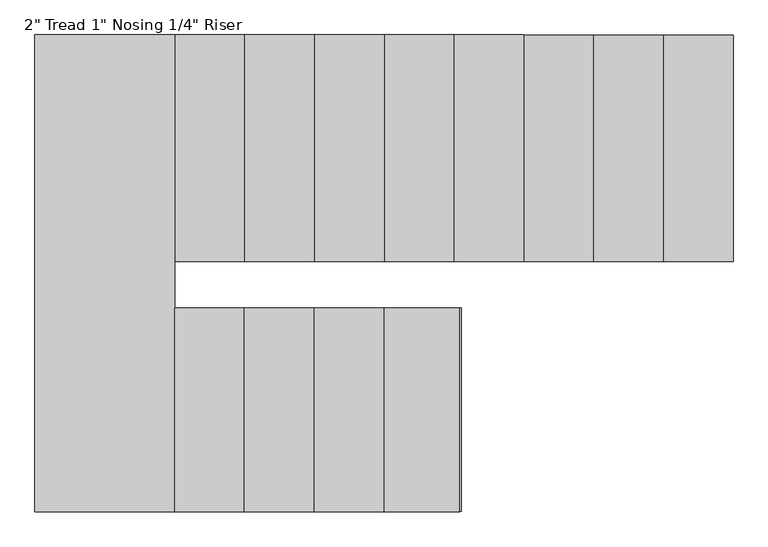
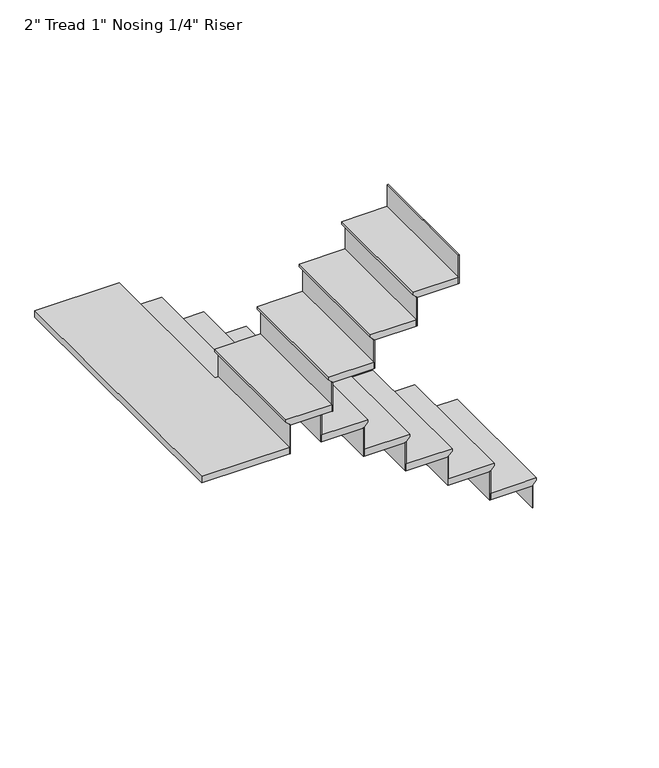
"""IFC4 building model written with IfcOpenShell, lengths in millimetres: stair flight geometry."""

from ifc_helpers import new_model, si_unit, origin, place, context, project, spatial, faceted_brep, source, transform, mapped, element, save


def stair_flight_46f16e2a(model_context):
    return source(origin(), model_context, "Body", "Brep", [
        faceted_brep([(-569.5630704, 657.3457979, 198.6642857), (-569.5630704, 657.3457979, 217.7142857), (-569.5630704, -333.2542021, 217.7142857), (-569.5630704, -333.2542021, 198.6642857), (-594.9630704, 657.3457979, 173.2642857), (-594.9630704, -333.2542021, 173.2642857), (-899.7630704, 657.3457979, 217.7142857), (-899.7630704, -333.2542021, 217.7142857), (-594.9630704, -333.2542021, 166.9142857), (-899.7630704, -333.2542021, 166.9142857), (-899.7630704, 657.3457979, 166.9142857), (-594.9630704, 657.3457979, 166.9142857)], [[[0, 1, 2, 3]], [[4, 0, 3, 5]], [[2, 1, 6, 7]], [[8, 9, 10, 11]], [[2, 7, 9, 8, 5, 3]], [[8, 11, 4, 5]], [[6, 1, 0, 4, 11, 10]], [[7, 6, 10, 9]]]),
        faceted_brep([(-594.9630704, 657.3457979, 166.9142857), (-594.9630704, 657.3457979, 0.0), (-601.3130704, 657.3457979, 0.0), (-601.3130704, 657.3457979, 166.9142857), (-594.9630704, -333.2542021, 166.9142857), (-601.3130704, -333.2542021, 166.9142857), (-601.3130704, -333.2542021, 0.0), (-594.9630704, -333.2542021, 0.0)], [[[0, 1, 2, 3]], [[4, 5, 6, 7]], [[1, 0, 4, 7]], [[2, 1, 7, 6]], [[3, 2, 6, 5]], [[0, 3, 5, 4]]]),
        faceted_brep([(-899.7630704, 657.3457979, 384.6285714), (-899.7630704, 657.3457979, 166.9142857), (-906.1130704, 657.3457979, 166.9142857), (-906.1130704, 657.3457979, 384.6285714), (-899.7630704, -333.2542021, 384.6285714), (-906.1130704, -333.2542021, 384.6285714), (-906.1130704, -333.2542021, 166.9142857), (-899.7630704, -333.2542021, 166.9142857)], [[[0, 1, 2, 3]], [[4, 5, 6, 7]], [[1, 0, 4, 7]], [[2, 1, 7, 6]], [[3, 2, 6, 5]], [[0, 3, 5, 4]]]),
        faceted_brep([(-874.3630704, -333.2542021, 435.4285714), (-874.3630704, 657.3457979, 435.4285714), (-1204.5630704, 657.3457979, 435.4285714), (-1204.5630704, -333.2542021, 435.4285714), (-899.7630704, -333.2542021, 384.6285714), (-1204.5630704, -333.2542021, 384.6285714), (-1204.5630704, 657.3457979, 384.6285714), (-899.7630704, 657.3457979, 384.6285714), (-899.7630704, -333.2542021, 390.9785714), (-874.3630704, -333.2542021, 416.3785714), (-899.7630704, 657.3457979, 390.9785714), (-874.3630704, 657.3457979, 416.3785714)], [[[0, 1, 2, 3]], [[4, 5, 6, 7]], [[0, 3, 5, 4, 8, 9]], [[4, 7, 10, 8]], [[2, 1, 11, 10, 7, 6]], [[3, 2, 6, 5]], [[11, 1, 0, 9]], [[10, 11, 9, 8]]]),
        faceted_brep([(-1204.5630704, 657.3457979, 602.3428571), (-1204.5630704, 657.3457979, 384.6285714), (-1210.9130704, 657.3457979, 384.6285714), (-1210.9130704, 657.3457979, 602.3428571), (-1204.5630704, -333.2542021, 602.3428571), (-1210.9130704, -333.2542021, 602.3428571), (-1210.9130704, -333.2542021, 384.6285714), (-1204.5630704, -333.2542021, 384.6285714)], [[[0, 1, 2, 3]], [[4, 5, 6, 7]], [[1, 0, 4, 7]], [[2, 1, 7, 6]], [[3, 2, 6, 5]], [[0, 3, 5, 4]]]),
        faceted_brep([(-1179.1630704, -333.2542021, 653.1428571), (-1179.1630704, 657.3457979, 653.1428571), (-1509.3630704, 657.3457979, 653.1428571), (-1509.3630704, -333.2542021, 653.1428571), (-1204.5630704, -333.2542021, 602.3428571), (-1509.3630704, -333.2542021, 602.3428571), (-1509.3630704, 657.3457979, 602.3428571), (-1204.5630704, 657.3457979, 602.3428571), (-1204.5630704, -333.2542021, 608.6928571), (-1179.1630704, -333.2542021, 634.0928571), (-1204.5630704, 657.3457979, 608.6928571), (-1179.1630704, 657.3457979, 634.0928571)], [[[0, 1, 2, 3]], [[4, 5, 6, 7]], [[0, 3, 5, 4, 8, 9]], [[4, 7, 10, 8]], [[2, 1, 11, 10, 7, 6]], [[3, 2, 6, 5]], [[11, 1, 0, 9]], [[10, 11, 9, 8]]]),
        faceted_brep([(-1509.3630704, 657.3457979, 820.0571429), (-1509.3630704, 657.3457979, 602.3428571), (-1515.7130704, 657.3457979, 602.3428571), (-1515.7130704, 657.3457979, 820.0571429), (-1509.3630704, -333.2542021, 820.0571429), (-1515.7130704, -333.2542021, 820.0571429), (-1515.7130704, -333.2542021, 602.3428571), (-1509.3630704, -333.2542021, 602.3428571)], [[[0, 1, 2, 3]], [[4, 5, 6, 7]], [[1, 0, 4, 7]], [[2, 1, 7, 6]], [[3, 2, 6, 5]], [[0, 3, 5, 4]]]),
        faceted_brep([(-1483.9630704, -333.2542021, 870.8571429), (-1483.9630704, 657.3457979, 870.8571429), (-1814.1630704, 657.3457979, 870.8571429), (-1814.1630704, -333.2542021, 870.8571429), (-1509.3630704, -333.2542021, 820.0571429), (-1814.1630704, -333.2542021, 820.0571429), (-1814.1630704, 657.3457979, 820.0571429), (-1509.3630704, 657.3457979, 820.0571429), (-1509.3630704, -333.2542021, 826.4071429), (-1483.9630704, -333.2542021, 851.8071429), (-1509.3630704, 657.3457979, 826.4071429), (-1483.9630704, 657.3457979, 851.8071429)], [[[0, 1, 2, 3]], [[4, 5, 6, 7]], [[0, 3, 5, 4, 8, 9]], [[4, 7, 10, 8]], [[2, 1, 11, 10, 7, 6]], [[3, 2, 6, 5]], [[11, 1, 0, 9]], [[10, 11, 9, 8]]]),
        faceted_brep([(-1814.1630704, 657.3457979, 1037.7714286), (-1814.1630704, 657.3457979, 820.0571429), (-1820.5130704, 657.3457979, 820.0571429), (-1820.5130704, 657.3457979, 1037.7714286), (-1814.1630704, -333.2542021, 1037.7714286), (-1820.5130704, -333.2542021, 1037.7714286), (-1820.5130704, -333.2542021, 820.0571429), (-1814.1630704, -333.2542021, 820.0571429)], [[[0, 1, 2, 3]], [[4, 5, 6, 7]], [[1, 0, 4, 7]], [[2, 1, 7, 6]], [[3, 2, 6, 5]], [[0, 3, 5, 4]]]),
        faceted_brep([(-1788.7630704, -333.2542021, 1088.5714286), (-1788.7630704, 657.3457979, 1088.5714286), (-2118.9630704, 657.3457979, 1088.5714286), (-2118.9630704, -333.2542021, 1088.5714286), (-1814.1630704, -333.2542021, 1037.7714286), (-2118.9630704, -333.2542021, 1037.7714286), (-2118.9630704, 657.3457979, 1037.7714286), (-1814.1630704, 657.3457979, 1037.7714286), (-1814.1630704, -333.2542021, 1044.1214286), (-1788.7630704, -333.2542021, 1069.5214286), (-1814.1630704, 657.3457979, 1044.1214286), (-1788.7630704, 657.3457979, 1069.5214286)], [[[0, 1, 2, 3]], [[4, 5, 6, 7]], [[0, 3, 5, 4, 8, 9]], [[4, 7, 10, 8]], [[2, 1, 11, 10, 7, 6]], [[3, 2, 6, 5]], [[11, 1, 0, 9]], [[10, 11, 9, 8]]]),
        faceted_brep([(-2118.9630704, 657.3457979, 1255.4857143), (-2118.9630704, 657.3457979, 1037.7714286), (-2125.3130704, 657.3457979, 1037.7714286), (-2125.3130704, 657.3457979, 1255.4857143), (-2118.9630704, -333.2542021, 1255.4857143), (-2125.3130704, -333.2542021, 1255.4857143), (-2125.3130704, -333.2542021, 1037.7714286), (-2118.9630704, -333.2542021, 1037.7714286)], [[[0, 1, 2, 3]], [[4, 5, 6, 7]], [[1, 0, 4, 7]], [[2, 1, 7, 6]], [[3, 2, 6, 5]], [[0, 3, 5, 4]]]),
        faceted_brep([(-2093.5630704, -333.2542021, 1306.2857143), (-2093.5630704, 657.3457979, 1306.2857143), (-2423.7630704, 657.3457979, 1306.2857143), (-2423.7630704, -333.2542021, 1306.2857143), (-2118.9630704, -333.2542021, 1255.4857143), (-2423.7630704, -333.2542021, 1255.4857143), (-2423.7630704, 657.3457979, 1255.4857143), (-2118.9630704, 657.3457979, 1255.4857143), (-2118.9630704, -333.2542021, 1261.8357143), (-2093.5630704, -333.2542021, 1287.2357143), (-2118.9630704, 657.3457979, 1261.8357143), (-2093.5630704, 657.3457979, 1287.2357143)], [[[0, 1, 2, 3]], [[4, 5, 6, 7]], [[0, 3, 5, 4, 8, 9]], [[4, 7, 10, 8]], [[2, 1, 11, 10, 7, 6]], [[3, 2, 6, 5]], [[11, 1, 0, 9]], [[10, 11, 9, 8]]]),
        faceted_brep([(-2423.7630704, 657.3457979, 1473.2), (-2423.7630704, 657.3457979, 1255.4857143), (-2430.1130704, 657.3457979, 1255.4857143), (-2430.1130704, 657.3457979, 1473.2), (-2423.7630704, -333.2542021, 1473.2), (-2430.1130704, -333.2542021, 1473.2), (-2430.1130704, -333.2542021, 1255.4857143), (-2423.7630704, -333.2542021, 1255.4857143)], [[[0, 1, 2, 3]], [[4, 5, 6, 7]], [[1, 0, 4, 7]], [[2, 1, 7, 6]], [[3, 2, 6, 5]], [[0, 3, 5, 4]]]),
        faceted_brep([(-2398.3630704, -333.2542021, 1524.0), (-2398.3630704, 657.3457979, 1524.0), (-2728.5630704, 657.3457979, 1524.0), (-2728.5630704, -333.2542021, 1524.0), (-2423.7630704, -333.2542021, 1473.2), (-2728.5630704, -333.2542021, 1473.2), (-2728.5630704, 657.3457979, 1473.2), (-2423.7630704, 657.3457979, 1473.2), (-2423.7630704, -333.2542021, 1479.55), (-2398.3630704, -333.2542021, 1504.95), (-2423.7630704, 657.3457979, 1479.55), (-2398.3630704, 657.3457979, 1504.95)], [[[0, 1, 2, 3]], [[4, 5, 6, 7]], [[0, 3, 5, 4, 8, 9]], [[4, 7, 10, 8]], [[2, 1, 11, 10, 7, 6]], [[3, 2, 6, 5]], [[11, 1, 0, 9]], [[10, 11, 9, 8]]]),
        faceted_brep([(-2728.5630704, 657.3457979, 1690.9142857), (-2728.5630704, 657.3457979, 1473.2), (-2734.9130704, 657.3457979, 1473.2), (-2734.9130704, 657.3457979, 1690.9142857), (-2728.5630704, -333.2542021, 1690.9142857), (-2734.9130704, -333.2542021, 1690.9142857), (-2734.9130704, -333.2542021, 1473.2), (-2728.5630704, -333.2542021, 1473.2)], [[[0, 1, 2, 3]], [[4, 5, 6, 7]], [[1, 0, 4, 7]], [[2, 1, 7, 6]], [[3, 2, 6, 5]], [[0, 3, 5, 4]]]),
        faceted_brep([(-2703.1630704, -333.2542021, 1741.7142857), (-2703.1630704, 657.3457979, 1741.7142857), (-3033.3630704, 657.3457979, 1741.7142857), (-3033.3630704, -333.2542021, 1741.7142857), (-2728.5630704, -333.2542021, 1690.9142857), (-3033.3630704, -333.2542021, 1690.9142857), (-3033.3630704, 657.3457979, 1690.9142857), (-2728.5630704, 657.3457979, 1690.9142857), (-2728.5630704, -333.2542021, 1697.2642857), (-2703.1630704, -333.2542021, 1722.6642857), (-2728.5630704, 657.3457979, 1697.2642857), (-2703.1630704, 657.3457979, 1722.6642857)], [[[0, 1, 2, 3]], [[4, 5, 6, 7]], [[0, 3, 5, 4, 8, 9]], [[4, 7, 10, 8]], [[2, 1, 11, 10, 7, 6]], [[3, 2, 6, 5]], [[11, 1, 0, 9]], [[10, 11, 9, 8]]]),
        faceted_brep([(-3033.3630704, 657.3457979, 1908.6285714), (-3033.3630704, 657.3457979, 1690.9142857), (-3039.7130704, 657.3457979, 1690.9142857), (-3039.7130704, 657.3457979, 1908.6285714), (-3033.3630704, -333.2542021, 1908.6285714), (-3039.7130704, -333.2542021, 1908.6285714), (-3039.7130704, -333.2542021, 1690.9142857), (-3033.3630704, -333.2542021, 1690.9142857)], [[[0, 1, 2, 3]], [[4, 5, 6, 7]], [[1, 0, 4, 7]], [[2, 1, 7, 6]], [[3, 2, 6, 5]], [[0, 3, 5, 4]]]),
        faceted_brep([(-2982.5630704, -536.4542021, 1959.4285714), (-3007.9630704, -536.4542021, 1959.4285714), (-3007.9630704, 657.3457979, 1959.4285714), (-3617.5630704, 657.3457979, 1959.4285714), (-3617.5630704, -1425.4542021, 1959.4285714), (-2982.5630704, -1425.4542021, 1959.4285714), (-3007.9630704, -536.4542021, 1908.6285714), (-2982.5630704, -536.4542021, 1908.6285714), (-2982.5630704, -1425.4542021, 1908.6285714), (-3617.5630704, -1425.4542021, 1908.6285714), (-3617.5630704, 657.3457979, 1908.6285714), (-3033.3630704, 657.3457979, 1908.6285714), (-3033.3630704, -333.2542021, 1908.6285714), (-3007.9630704, -333.2542021, 1908.6285714), (-3007.9630704, -333.2542021, 1940.3785714), (-3007.9630704, 657.3457979, 1940.3785714), (-3033.3630704, -333.2542021, 1914.9785714), (-3033.3630704, 657.3457979, 1914.9785714)], [[[0, 1, 2, 3, 4, 5]], [[6, 7, 8, 9, 10, 11, 12, 13]], [[1, 0, 7, 6]], [[2, 1, 6, 13, 14, 15]], [[13, 12, 16, 14]], [[12, 11, 17, 16]], [[3, 2, 15, 17, 11, 10]], [[4, 3, 10, 9]], [[5, 4, 9, 8]], [[0, 5, 8, 7]], [[17, 15, 14, 16]]]),
        faceted_brep([(-2982.5630704, -1425.4542021, 2126.3428571), (-2982.5630704, -1425.4542021, 1908.6285714), (-2976.2130704, -1425.4542021, 1908.6285714), (-2976.2130704, -1425.4542021, 2126.3428571), (-2982.5630704, -536.4542021, 2126.3428571), (-2976.2130704, -536.4542021, 2126.3428571), (-2976.2130704, -536.4542021, 1908.6285714), (-2982.5630704, -536.4542021, 1908.6285714)], [[[0, 1, 2, 3]], [[4, 5, 6, 7]], [[1, 0, 4, 7]], [[2, 1, 7, 6]], [[3, 2, 6, 5]], [[0, 3, 5, 4]]]),
        faceted_brep([(-3007.9630704, -536.4542021, 2177.1428571), (-3007.9630704, -1425.4542021, 2177.1428571), (-2677.7630704, -1425.4542021, 2177.1428571), (-2677.7630704, -536.4542021, 2177.1428571), (-2982.5630704, -536.4542021, 2126.3428571), (-2677.7630704, -536.4542021, 2126.3428571), (-2677.7630704, -1425.4542021, 2126.3428571), (-2982.5630704, -1425.4542021, 2126.3428571), (-2982.5630704, -536.4542021, 2132.6928571), (-3007.9630704, -536.4542021, 2158.0928571), (-2982.5630704, -1425.4542021, 2132.6928571), (-3007.9630704, -1425.4542021, 2158.0928571)], [[[0, 1, 2, 3]], [[4, 5, 6, 7]], [[0, 3, 5, 4, 8, 9]], [[4, 7, 10, 8]], [[2, 1, 11, 10, 7, 6]], [[3, 2, 6, 5]], [[11, 1, 0, 9]], [[10, 11, 9, 8]]]),
        faceted_brep([(-2677.7630704, -1425.4542021, 2344.0571429), (-2677.7630704, -1425.4542021, 2126.3428571), (-2671.4130704, -1425.4542021, 2126.3428571), (-2671.4130704, -1425.4542021, 2344.0571429), (-2677.7630704, -536.4542021, 2344.0571429), (-2671.4130704, -536.4542021, 2344.0571429), (-2671.4130704, -536.4542021, 2126.3428571), (-2677.7630704, -536.4542021, 2126.3428571)], [[[0, 1, 2, 3]], [[4, 5, 6, 7]], [[1, 0, 4, 7]], [[2, 1, 7, 6]], [[3, 2, 6, 5]], [[0, 3, 5, 4]]]),
        faceted_brep([(-2703.1630704, -536.4542021, 2394.8571429), (-2703.1630704, -1425.4542021, 2394.8571429), (-2372.9630704, -1425.4542021, 2394.8571429), (-2372.9630704, -536.4542021, 2394.8571429), (-2677.7630704, -536.4542021, 2344.0571429), (-2372.9630704, -536.4542021, 2344.0571429), (-2372.9630704, -1425.4542021, 2344.0571429), (-2677.7630704, -1425.4542021, 2344.0571429), (-2677.7630704, -536.4542021, 2350.4071429), (-2703.1630704, -536.4542021, 2375.8071429), (-2677.7630704, -1425.4542021, 2350.4071429), (-2703.1630704, -1425.4542021, 2375.8071429)], [[[0, 1, 2, 3]], [[4, 5, 6, 7]], [[0, 3, 5, 4, 8, 9]], [[4, 7, 10, 8]], [[2, 1, 11, 10, 7, 6]], [[3, 2, 6, 5]], [[11, 1, 0, 9]], [[10, 11, 9, 8]]]),
        faceted_brep([(-2372.9630704, -1425.4542021, 2561.7714286), (-2372.9630704, -1425.4542021, 2344.0571429), (-2366.6130704, -1425.4542021, 2344.0571429), (-2366.6130704, -1425.4542021, 2561.7714286), (-2372.9630704, -536.4542021, 2561.7714286), (-2366.6130704, -536.4542021, 2561.7714286), (-2366.6130704, -536.4542021, 2344.0571429), (-2372.9630704, -536.4542021, 2344.0571429)], [[[0, 1, 2, 3]], [[4, 5, 6, 7]], [[1, 0, 4, 7]], [[2, 1, 7, 6]], [[3, 2, 6, 5]], [[0, 3, 5, 4]]]),
        faceted_brep([(-2398.3630704, -536.4542021, 2612.5714286), (-2398.3630704, -1425.4542021, 2612.5714286), (-2068.1630704, -1425.4542021, 2612.5714286), (-2068.1630704, -536.4542021, 2612.5714286), (-2372.9630704, -536.4542021, 2561.7714286), (-2068.1630704, -536.4542021, 2561.7714286), (-2068.1630704, -1425.4542021, 2561.7714286), (-2372.9630704, -1425.4542021, 2561.7714286), (-2372.9630704, -536.4542021, 2568.1214286), (-2398.3630704, -536.4542021, 2593.5214286), (-2372.9630704, -1425.4542021, 2568.1214286), (-2398.3630704, -1425.4542021, 2593.5214286)], [[[0, 1, 2, 3]], [[4, 5, 6, 7]], [[0, 3, 5, 4, 8, 9]], [[4, 7, 10, 8]], [[2, 1, 11, 10, 7, 6]], [[3, 2, 6, 5]], [[11, 1, 0, 9]], [[10, 11, 9, 8]]]),
        faceted_brep([(-2068.1630704, -1425.4542021, 2779.4857143), (-2068.1630704, -1425.4542021, 2561.7714286), (-2061.8130704, -1425.4542021, 2561.7714286), (-2061.8130704, -1425.4542021, 2779.4857143), (-2068.1630704, -536.4542021, 2779.4857143), (-2061.8130704, -536.4542021, 2779.4857143), (-2061.8130704, -536.4542021, 2561.7714286), (-2068.1630704, -536.4542021, 2561.7714286)], [[[0, 1, 2, 3]], [[4, 5, 6, 7]], [[1, 0, 4, 7]], [[2, 1, 7, 6]], [[3, 2, 6, 5]], [[0, 3, 5, 4]]]),
        faceted_brep([(-1763.3630704, -1425.4542021, 2997.2), (-1763.3630704, -1425.4542021, 2779.4857143), (-1757.0130704, -1425.4542021, 2779.4857143), (-1757.0130704, -1425.4542021, 2997.2), (-1763.3630704, -536.4542021, 2997.2), (-1757.0130704, -536.4542021, 2997.2), (-1757.0130704, -536.4542021, 2779.4857143), (-1763.3630704, -536.4542021, 2779.4857143)], [[[0, 1, 2, 3]], [[4, 5, 6, 7]], [[1, 0, 4, 7]], [[2, 1, 7, 6]], [[3, 2, 6, 5]], [[0, 3, 5, 4]]]),
        faceted_brep([(-2093.5630704, -536.4542021, 2830.2857143), (-2093.5630704, -1425.4542021, 2830.2857143), (-1763.3630704, -1425.4542021, 2830.2857143), (-1763.3630704, -536.4542021, 2830.2857143), (-2068.1630704, -536.4542021, 2779.4857143), (-1763.3630704, -536.4542021, 2779.4857143), (-1763.3630704, -1425.4542021, 2779.4857143), (-2068.1630704, -1425.4542021, 2779.4857143), (-2068.1630704, -536.4542021, 2785.8357143), (-2093.5630704, -536.4542021, 2811.2357143), (-2068.1630704, -1425.4542021, 2785.8357143), (-2093.5630704, -1425.4542021, 2811.2357143)], [[[0, 1, 2, 3]], [[4, 5, 6, 7]], [[0, 3, 5, 4, 8, 9]], [[4, 7, 10, 8]], [[2, 1, 11, 10, 7, 6]], [[3, 2, 6, 5]], [[11, 1, 0, 9]], [[10, 11, 9, 8]]]),
    ])


if __name__ == "__main__":
    model = new_model("IFC4")
    model_context = context("Model", 3, world=origin())
    ifc_project = project(units=[si_unit("LENGTHUNIT", "METRE", prefix="MILLI")], contexts=[model_context])
    site = spatial("IfcSite", under=ifc_project)
    building = spatial("IfcBuilding", under=site)
    placement = place(None, origin())
    stair_flight_shape = stair_flight_46f16e2a(model_context)
    element("IfcStairFlight", 1, ObjectType="2\" Tread 1\" Nosing 1/4\" Riser", at=placement, inside=building, context=model_context, shape_type="MappedRepresentation", body=[
        mapped(stair_flight_shape, transform((0.0, 0.0, 0.0), x_axis=(1.0, 0.0, 0.0), y_axis=(0.0, 1.0, 0.0), z_axis=(0.0, 0.0, 1.0))),
    ])
    save(model, "model.ifc")
